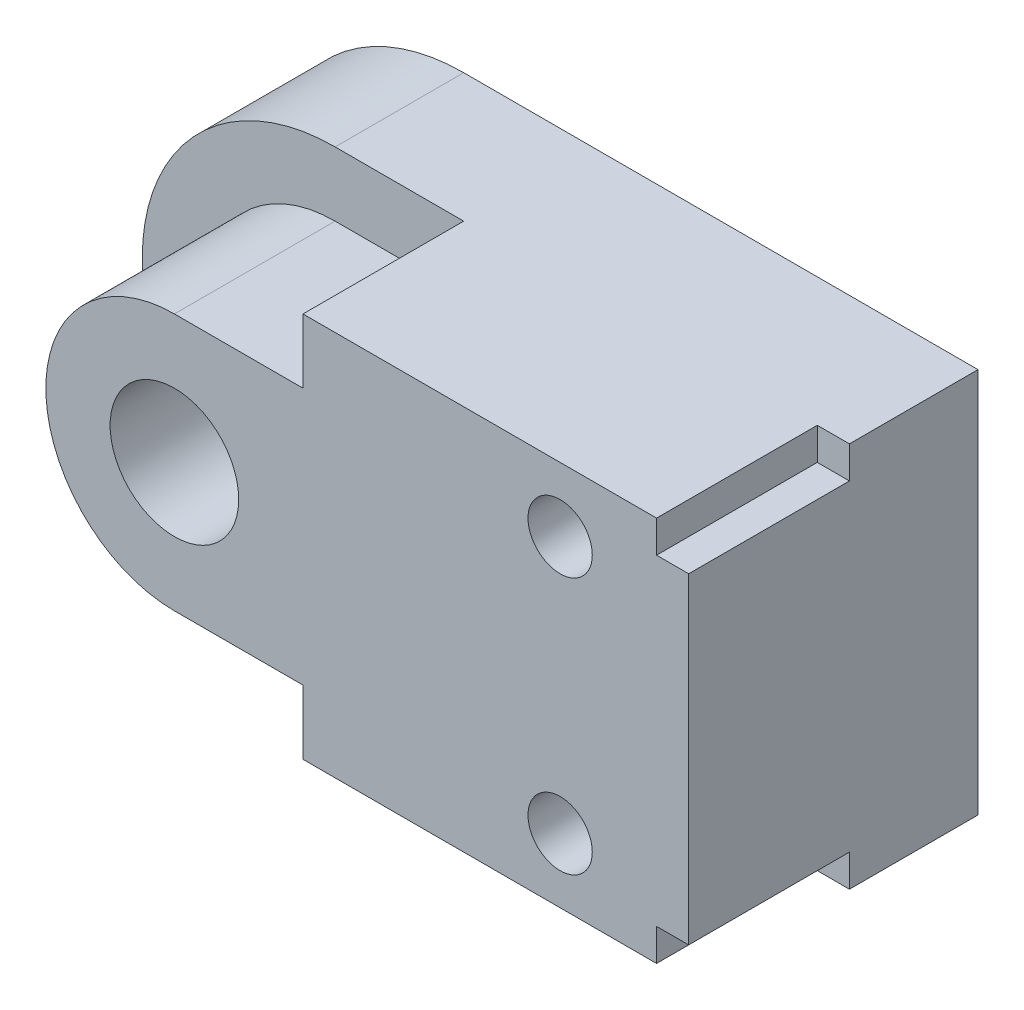
ISO-10303-21;
HEADER;
FILE_DESCRIPTION(('STEP AP214'),'2;1');
FILE_NAME('part.step','',(''),(''),'','','');
FILE_SCHEMA(('AUTOMOTIVE_DESIGN { 1 0 10303 214 1 1 1 1 }'));
ENDSEC;
DATA;
#1=APPLICATION_CONTEXT('core data for automotive mechanical design processes');
#2=APPLICATION_PROTOCOL_DEFINITION('international standard','automotive_design',2000,#1);
#3=PRODUCT_CONTEXT('',#1,'mechanical');
#4=PRODUCT('Part','Part','',(#3));
#5=PRODUCT_RELATED_PRODUCT_CATEGORY('part','',(#4));
#6=PRODUCT_DEFINITION_FORMATION('','',#4);
#7=PRODUCT_DEFINITION_CONTEXT('part definition',#1,'design');
#8=PRODUCT_DEFINITION('design','',#6,#7);
#9=PRODUCT_DEFINITION_SHAPE('','',#8);
#10=(LENGTH_UNIT() NAMED_UNIT(*) SI_UNIT(.MILLI.,.METRE.));
#11=(NAMED_UNIT(*) PLANE_ANGLE_UNIT() SI_UNIT($,.RADIAN.));
#12=(NAMED_UNIT(*) SI_UNIT($,.STERADIAN.) SOLID_ANGLE_UNIT());
#13=UNCERTAINTY_MEASURE_WITH_UNIT(LENGTH_MEASURE(1.E-05),#10,'distance_accuracy_value','');
#14=(GEOMETRIC_REPRESENTATION_CONTEXT(3) GLOBAL_UNCERTAINTY_ASSIGNED_CONTEXT((#13)) GLOBAL_UNIT_ASSIGNED_CONTEXT((#10,
#11,#12)) REPRESENTATION_CONTEXT('',''));
#15=CARTESIAN_POINT('',(0.,0.,0.));
#16=DIRECTION('',(0.,0.,1.));
#17=DIRECTION('',(1.,0.,0.));
#18=AXIS2_PLACEMENT_3D('',#15,#16,#17);
#19=CARTESIAN_POINT('',(0.,0.,20.));
#20=DIRECTION('',(0.,0.,1.));
#21=DIRECTION('',(1.,0.,0.));
#22=AXIS2_PLACEMENT_3D('',#19,#20,#21);
#23=PLANE('',#22);
#24=DIRECTION('',(0.,1.,0.));
#25=VECTOR('',#24,1.);
#26=CARTESIAN_POINT('',(75.,30.,20.));
#27=LINE('',#26,#25);
#28=CARTESIAN_POINT('',(75.,25.,20.));
#29=VERTEX_POINT('',#28);
#30=CARTESIAN_POINT('',(75.,30.,20.));
#31=VERTEX_POINT('',#30);
#32=EDGE_CURVE('E53',#29,#31,#27,.T.);
#33=ORIENTED_EDGE('',*,*,#32,.F.);
#34=DIRECTION('',(-1.,0.,0.));
#35=VECTOR('',#34,1.);
#36=CARTESIAN_POINT('',(80.,25.,20.));
#37=LINE('',#36,#35);
#38=CARTESIAN_POINT('',(80.,25.,20.));
#39=VERTEX_POINT('',#38);
#40=EDGE_CURVE('E288',#39,#29,#37,.T.);
#41=ORIENTED_EDGE('',*,*,#40,.F.);
#42=DIRECTION('',(0.,1.,0.));
#43=VECTOR('',#42,1.);
#44=CARTESIAN_POINT('',(80.,30.,20.));
#45=LINE('',#44,#43);
#46=CARTESIAN_POINT('',(80.,30.,20.));
#47=VERTEX_POINT('',#46);
#48=EDGE_CURVE('E193',#39,#47,#45,.T.);
#49=ORIENTED_EDGE('',*,*,#48,.T.);
#50=DIRECTION('',(-1.,0.,0.));
#51=VECTOR('',#50,1.);
#52=CARTESIAN_POINT('',(0.,30.,20.));
#53=LINE('',#52,#51);
#54=EDGE_CURVE('E196',#47,#31,#53,.T.);
#55=ORIENTED_EDGE('',*,*,#54,.T.);
#56=EDGE_LOOP('',(#33,#41,#49,#55));
#57=FACE_BOUND('',#56,.T.);
#58=ADVANCED_FACE('F39',(#57),#23,.T.);
#59=DIRECTION('',(1.,0.,0.));
#60=VECTOR('',#59,1.);
#61=CARTESIAN_POINT('',(80.,-25.,20.));
#62=LINE('',#61,#60);
#63=CARTESIAN_POINT('',(75.,-25.,20.));
#64=VERTEX_POINT('',#63);
#65=CARTESIAN_POINT('',(80.,-25.,20.));
#66=VERTEX_POINT('',#65);
#67=EDGE_CURVE('E64',#64,#66,#62,.T.);
#68=ORIENTED_EDGE('',*,*,#67,.F.);
#69=DIRECTION('',(0.,1.,0.));
#70=VECTOR('',#69,1.);
#71=CARTESIAN_POINT('',(75.,-30.,20.));
#72=LINE('',#71,#70);
#73=CARTESIAN_POINT('',(75.,-30.,20.));
#74=VERTEX_POINT('',#73);
#75=EDGE_CURVE('E283',#74,#64,#72,.T.);
#76=ORIENTED_EDGE('',*,*,#75,.F.);
#77=DIRECTION('',(1.,0.,0.));
#78=VECTOR('',#77,1.);
#79=CARTESIAN_POINT('',(80.,-30.,20.));
#80=LINE('',#79,#78);
#81=CARTESIAN_POINT('',(80.,-30.,20.));
#82=VERTEX_POINT('',#81);
#83=EDGE_CURVE('E186',#74,#82,#80,.T.);
#84=ORIENTED_EDGE('',*,*,#83,.T.);
#85=EDGE_CURVE('E192',#82,#66,#45,.T.);
#86=ORIENTED_EDGE('',*,*,#85,.T.);
#87=EDGE_LOOP('',(#68,#76,#84,#86));
#88=FACE_BOUND('',#87,.T.);
#89=ADVANCED_FACE('F340',(#88),#23,.T.);
#90=DIRECTION('',(0.,-1.,0.));
#91=VECTOR('',#90,1.);
#92=CARTESIAN_POINT('',(20.,20.,20.));
#93=LINE('',#92,#91);
#94=CARTESIAN_POINT('',(20.,30.,20.));
#95=VERTEX_POINT('',#94);
#96=CARTESIAN_POINT('',(20.,20.,20.));
#97=VERTEX_POINT('',#96);
#98=EDGE_CURVE('E239',#95,#97,#93,.T.);
#99=ORIENTED_EDGE('',*,*,#98,.F.);
#100=CARTESIAN_POINT('',(0.,30.,20.));
#101=VERTEX_POINT('',#100);
#102=EDGE_CURVE('E197',#95,#101,#53,.T.);
#103=ORIENTED_EDGE('',*,*,#102,.T.);
#104=CARTESIAN_POINT('',(0.,0.,20.));
#105=DIRECTION('',(0.,0.,1.));
#106=DIRECTION('',(1.,0.,0.));
#107=AXIS2_PLACEMENT_3D('',#104,#105,#106);
#108=CIRCLE('',#107,30.);
#109=CARTESIAN_POINT('',(0.,-30.,20.));
#110=VERTEX_POINT('',#109);
#111=EDGE_CURVE('E189',#101,#110,#108,.T.);
#112=ORIENTED_EDGE('',*,*,#111,.T.);
#113=CARTESIAN_POINT('',(20.,-30.,20.));
#114=VERTEX_POINT('',#113);
#115=EDGE_CURVE('E191',#110,#114,#80,.T.);
#116=ORIENTED_EDGE('',*,*,#115,.T.);
#117=DIRECTION('',(0.,-1.,0.));
#118=VECTOR('',#117,1.);
#119=CARTESIAN_POINT('',(20.,-30.,20.));
#120=LINE('',#119,#118);
#121=CARTESIAN_POINT('',(20.,-20.,20.));
#122=VERTEX_POINT('',#121);
#123=EDGE_CURVE('E278',#122,#114,#120,.T.);
#124=ORIENTED_EDGE('',*,*,#123,.F.);
#125=DIRECTION('',(1.,0.,0.));
#126=VECTOR('',#125,1.);
#127=CARTESIAN_POINT('',(20.,-20.,20.));
#128=LINE('',#127,#126);
#129=CARTESIAN_POINT('',(0.,-20.,20.));
#130=VERTEX_POINT('',#129);
#131=EDGE_CURVE('E284',#130,#122,#128,.T.);
#132=ORIENTED_EDGE('',*,*,#131,.F.);
#133=CARTESIAN_POINT('',(0.,0.,20.));
#134=DIRECTION('',(0.,0.,1.));
#135=DIRECTION('',(1.,0.,0.));
#136=AXIS2_PLACEMENT_3D('',#133,#134,#135);
#137=CIRCLE('',#136,20.);
#138=CARTESIAN_POINT('',(0.,20.,20.));
#139=VERTEX_POINT('',#138);
#140=EDGE_CURVE('E176',#139,#130,#137,.T.);
#141=ORIENTED_EDGE('',*,*,#140,.F.);
#142=DIRECTION('',(-1.,0.,0.));
#143=VECTOR('',#142,1.);
#144=CARTESIAN_POINT('',(0.,20.,20.));
#145=LINE('',#144,#143);
#146=EDGE_CURVE('E175',#97,#139,#145,.T.);
#147=ORIENTED_EDGE('',*,*,#146,.F.);
#148=EDGE_LOOP('',(#99,#103,#112,#116,#124,#132,#141,#147));
#149=FACE_BOUND('',#148,.T.);
#150=ADVANCED_FACE('F237',(#149),#23,.T.);
#151=CARTESIAN_POINT('',(0.,0.,0.));
#152=DIRECTION('',(0.,0.,1.));
#153=DIRECTION('',(1.,0.,0.));
#154=AXIS2_PLACEMENT_3D('',#151,#152,#153);
#155=PLANE('',#154);
#156=CARTESIAN_POINT('',(60.,-20.,0.));
#157=DIRECTION('',(0.,0.,1.));
#158=DIRECTION('',(1.,0.,0.));
#159=AXIS2_PLACEMENT_3D('',#156,#157,#158);
#160=CIRCLE('',#159,5.);
#161=CARTESIAN_POINT('',(65.,-20.,0.));
#162=VERTEX_POINT('',#161);
#163=EDGE_CURVE('E540',#162,#162,#160,.T.);
#164=ORIENTED_EDGE('',*,*,#163,.T.);
#165=EDGE_LOOP('',(#164));
#166=FACE_BOUND('',#165,.T.);
#167=CARTESIAN_POINT('',(60.,20.,0.));
#168=DIRECTION('',(0.,0.,1.));
#169=DIRECTION('',(1.,0.,0.));
#170=AXIS2_PLACEMENT_3D('',#167,#168,#169);
#171=CIRCLE('',#170,5.);
#172=CARTESIAN_POINT('',(65.,20.,0.));
#173=VERTEX_POINT('',#172);
#174=EDGE_CURVE('E538',#173,#173,#171,.T.);
#175=ORIENTED_EDGE('',*,*,#174,.T.);
#176=EDGE_LOOP('',(#175));
#177=FACE_BOUND('',#176,.T.);
#178=CARTESIAN_POINT('',(0.,0.,0.));
#179=DIRECTION('',(0.,0.,1.));
#180=DIRECTION('',(1.,0.,0.));
#181=AXIS2_PLACEMENT_3D('',#178,#179,#180);
#182=CIRCLE('',#181,30.);
#183=CARTESIAN_POINT('',(0.,30.,0.));
#184=VERTEX_POINT('',#183);
#185=CARTESIAN_POINT('',(0.,-30.,0.));
#186=VERTEX_POINT('',#185);
#187=EDGE_CURVE('E182',#184,#186,#182,.T.);
#188=ORIENTED_EDGE('',*,*,#187,.F.);
#189=DIRECTION('',(-1.,0.,0.));
#190=VECTOR('',#189,1.);
#191=CARTESIAN_POINT('',(0.,30.,0.));
#192=LINE('',#191,#190);
#193=CARTESIAN_POINT('',(80.,30.,0.));
#194=VERTEX_POINT('',#193);
#195=EDGE_CURVE('E194',#194,#184,#192,.T.);
#196=ORIENTED_EDGE('',*,*,#195,.F.);
#197=DIRECTION('',(0.,1.,0.));
#198=VECTOR('',#197,1.);
#199=CARTESIAN_POINT('',(80.,30.,0.));
#200=LINE('',#199,#198);
#201=CARTESIAN_POINT('',(80.,-30.,0.));
#202=VERTEX_POINT('',#201);
#203=EDGE_CURVE('E202',#202,#194,#200,.T.);
#204=ORIENTED_EDGE('',*,*,#203,.F.);
#205=DIRECTION('',(1.,0.,0.));
#206=VECTOR('',#205,1.);
#207=CARTESIAN_POINT('',(80.,-30.,0.));
#208=LINE('',#207,#206);
#209=EDGE_CURVE('E201',#186,#202,#208,.T.);
#210=ORIENTED_EDGE('',*,*,#209,.F.);
#211=EDGE_LOOP('',(#188,#196,#204,#210));
#212=FACE_BOUND('',#211,.T.);
#213=CARTESIAN_POINT('',(0.,0.,0.));
#214=DIRECTION('',(0.,0.,1.));
#215=DIRECTION('',(1.,0.,0.));
#216=AXIS2_PLACEMENT_3D('',#213,#214,#215);
#217=CIRCLE('',#216,10.);
#218=CARTESIAN_POINT('',(10.,0.,0.));
#219=VERTEX_POINT('',#218);
#220=EDGE_CURVE('E180',#219,#219,#217,.T.);
#221=ORIENTED_EDGE('',*,*,#220,.T.);
#222=EDGE_LOOP('',(#221));
#223=FACE_BOUND('',#222,.T.);
#224=ADVANCED_FACE('F223',(#166,#177,#212,#223),#155,.F.);
#225=CARTESIAN_POINT('',(0.,0.,20.));
#226=DIRECTION('',(0.,0.,-1.));
#227=DIRECTION('',(-1.,0.,0.));
#228=AXIS2_PLACEMENT_3D('',#225,#226,#227);
#229=CYLINDRICAL_SURFACE('',#228,30.);
#230=ORIENTED_EDGE('',*,*,#187,.T.);
#231=DIRECTION('',(0.,0.,-1.));
#232=VECTOR('',#231,1.);
#233=CARTESIAN_POINT('',(0.,-30.,20.));
#234=LINE('',#233,#232);
#235=EDGE_CURVE('E11',#110,#186,#234,.T.);
#236=ORIENTED_EDGE('',*,*,#235,.F.);
#237=ORIENTED_EDGE('',*,*,#111,.F.);
#238=DIRECTION('',(0.,0.,-1.));
#239=VECTOR('',#238,1.);
#240=CARTESIAN_POINT('',(0.,30.,20.));
#241=LINE('',#240,#239);
#242=EDGE_CURVE('E199',#101,#184,#241,.T.);
#243=ORIENTED_EDGE('',*,*,#242,.T.);
#244=EDGE_LOOP('',(#230,#236,#237,#243));
#245=FACE_BOUND('',#244,.T.);
#246=ADVANCED_FACE('F41',(#245),#229,.T.);
#247=CARTESIAN_POINT('',(80.,-30.,20.));
#248=DIRECTION('',(0.,1.,0.));
#249=DIRECTION('',(-1.,0.,0.));
#250=AXIS2_PLACEMENT_3D('',#247,#248,#249);
#251=PLANE('',#250);
#252=ORIENTED_EDGE('',*,*,#209,.T.);
#253=DIRECTION('',(0.,0.,-1.));
#254=VECTOR('',#253,1.);
#255=CARTESIAN_POINT('',(80.,-30.,20.));
#256=LINE('',#255,#254);
#257=EDGE_CURVE('E50',#82,#202,#256,.T.);
#258=ORIENTED_EDGE('',*,*,#257,.F.);
#259=ORIENTED_EDGE('',*,*,#83,.F.);
#260=DIRECTION('',(0.,0.,-1.));
#261=VECTOR('',#260,1.);
#262=CARTESIAN_POINT('',(75.,-30.,45.));
#263=LINE('',#262,#261);
#264=CARTESIAN_POINT('',(75.,-30.,45.));
#265=VERTEX_POINT('',#264);
#266=EDGE_CURVE('E269',#265,#74,#263,.T.);
#267=ORIENTED_EDGE('',*,*,#266,.F.);
#268=DIRECTION('',(1.,0.,0.));
#269=VECTOR('',#268,1.);
#270=CARTESIAN_POINT('',(75.,-30.,45.));
#271=LINE('',#270,#269);
#272=CARTESIAN_POINT('',(20.,-30.,45.));
#273=VERTEX_POINT('',#272);
#274=EDGE_CURVE('E280',#273,#265,#271,.T.);
#275=ORIENTED_EDGE('',*,*,#274,.F.);
#276=DIRECTION('',(0.,0.,-1.));
#277=VECTOR('',#276,1.);
#278=CARTESIAN_POINT('',(20.,-30.,45.));
#279=LINE('',#278,#277);
#280=EDGE_CURVE('E181',#273,#114,#279,.T.);
#281=ORIENTED_EDGE('',*,*,#280,.T.);
#282=ORIENTED_EDGE('',*,*,#115,.F.);
#283=ORIENTED_EDGE('',*,*,#235,.T.);
#284=EDGE_LOOP('',(#252,#258,#259,#267,#275,#281,#282,#283));
#285=FACE_BOUND('',#284,.T.);
#286=ADVANCED_FACE('F274',(#285),#251,.F.);
#287=CARTESIAN_POINT('',(80.,30.,20.));
#288=DIRECTION('',(-1.,0.,0.));
#289=DIRECTION('',(0.,0.,1.));
#290=AXIS2_PLACEMENT_3D('',#287,#288,#289);
#291=PLANE('',#290);
#292=ORIENTED_EDGE('',*,*,#203,.T.);
#293=DIRECTION('',(0.,0.,-1.));
#294=VECTOR('',#293,1.);
#295=CARTESIAN_POINT('',(80.,30.,20.));
#296=LINE('',#295,#294);
#297=EDGE_CURVE('E209',#47,#194,#296,.T.);
#298=ORIENTED_EDGE('',*,*,#297,.F.);
#299=ORIENTED_EDGE('',*,*,#48,.F.);
#300=DIRECTION('',(0.,0.,-1.));
#301=VECTOR('',#300,1.);
#302=CARTESIAN_POINT('',(80.,25.,45.));
#303=LINE('',#302,#301);
#304=CARTESIAN_POINT('',(80.,25.,45.));
#305=VERTEX_POINT('',#304);
#306=EDGE_CURVE('E265',#305,#39,#303,.T.);
#307=ORIENTED_EDGE('',*,*,#306,.F.);
#308=DIRECTION('',(0.,1.,0.));
#309=VECTOR('',#308,1.);
#310=CARTESIAN_POINT('',(80.,25.,45.));
#311=LINE('',#310,#309);
#312=CARTESIAN_POINT('',(80.,-25.,45.));
#313=VERTEX_POINT('',#312);
#314=EDGE_CURVE('E312',#313,#305,#311,.T.);
#315=ORIENTED_EDGE('',*,*,#314,.F.);
#316=DIRECTION('',(0.,0.,-1.));
#317=VECTOR('',#316,1.);
#318=CARTESIAN_POINT('',(80.,-25.,45.));
#319=LINE('',#318,#317);
#320=EDGE_CURVE('E264',#313,#66,#319,.T.);
#321=ORIENTED_EDGE('',*,*,#320,.T.);
#322=ORIENTED_EDGE('',*,*,#85,.F.);
#323=ORIENTED_EDGE('',*,*,#257,.T.);
#324=EDGE_LOOP('',(#292,#298,#299,#307,#315,#321,#322,#323));
#325=FACE_BOUND('',#324,.T.);
#326=ADVANCED_FACE('F220',(#325),#291,.F.);
#327=CARTESIAN_POINT('',(0.,30.,20.));
#328=DIRECTION('',(0.,-1.,0.));
#329=DIRECTION('',(1.,0.,0.));
#330=AXIS2_PLACEMENT_3D('',#327,#328,#329);
#331=PLANE('',#330);
#332=ORIENTED_EDGE('',*,*,#195,.T.);
#333=ORIENTED_EDGE('',*,*,#242,.F.);
#334=ORIENTED_EDGE('',*,*,#102,.F.);
#335=DIRECTION('',(0.,0.,-1.));
#336=VECTOR('',#335,1.);
#337=CARTESIAN_POINT('',(20.,30.,45.));
#338=LINE('',#337,#336);
#339=CARTESIAN_POINT('',(20.,30.,45.));
#340=VERTEX_POINT('',#339);
#341=EDGE_CURVE('E242',#340,#95,#338,.T.);
#342=ORIENTED_EDGE('',*,*,#341,.F.);
#343=DIRECTION('',(-1.,0.,0.));
#344=VECTOR('',#343,1.);
#345=CARTESIAN_POINT('',(20.,30.,45.));
#346=LINE('',#345,#344);
#347=CARTESIAN_POINT('',(75.,30.,45.));
#348=VERTEX_POINT('',#347);
#349=EDGE_CURVE('E293',#348,#340,#346,.T.);
#350=ORIENTED_EDGE('',*,*,#349,.F.);
#351=DIRECTION('',(0.,0.,-1.));
#352=VECTOR('',#351,1.);
#353=CARTESIAN_POINT('',(75.,30.,45.));
#354=LINE('',#353,#352);
#355=EDGE_CURVE('E247',#348,#31,#354,.T.);
#356=ORIENTED_EDGE('',*,*,#355,.T.);
#357=ORIENTED_EDGE('',*,*,#54,.F.);
#358=ORIENTED_EDGE('',*,*,#297,.T.);
#359=EDGE_LOOP('',(#332,#333,#334,#342,#350,#356,#357,#358));
#360=FACE_BOUND('',#359,.T.);
#361=ADVANCED_FACE('F230',(#360),#331,.F.);
#362=CARTESIAN_POINT('',(0.,0.,20.));
#363=DIRECTION('',(0.,0.,-1.));
#364=DIRECTION('',(-1.,0.,0.));
#365=AXIS2_PLACEMENT_3D('',#362,#363,#364);
#366=CYLINDRICAL_SURFACE('',#365,10.);
#367=ORIENTED_EDGE('',*,*,#220,.F.);
#368=EDGE_LOOP('',(#367));
#369=FACE_BOUND('',#368,.T.);
#370=CARTESIAN_POINT('',(0.,0.,45.));
#371=DIRECTION('',(0.,0.,1.));
#372=DIRECTION('',(1.,0.,0.));
#373=AXIS2_PLACEMENT_3D('',#370,#371,#372);
#374=CIRCLE('',#373,10.);
#375=CARTESIAN_POINT('',(10.,0.,45.));
#376=VERTEX_POINT('',#375);
#377=EDGE_CURVE('E297',#376,#376,#374,.T.);
#378=ORIENTED_EDGE('',*,*,#377,.T.);
#379=EDGE_LOOP('',(#378));
#380=FACE_BOUND('',#379,.T.);
#381=ADVANCED_FACE('F346',(#369,#380),#366,.F.);
#382=CARTESIAN_POINT('',(0.,0.,45.));
#383=DIRECTION('',(0.,0.,1.));
#384=DIRECTION('',(1.,0.,0.));
#385=AXIS2_PLACEMENT_3D('',#382,#383,#384);
#386=PLANE('',#385);
#387=CARTESIAN_POINT('',(60.,20.,45.));
#388=DIRECTION('',(0.,0.,1.));
#389=DIRECTION('',(1.,0.,0.));
#390=AXIS2_PLACEMENT_3D('',#387,#388,#389);
#391=CIRCLE('',#390,5.);
#392=CARTESIAN_POINT('',(65.,20.,45.));
#393=VERTEX_POINT('',#392);
#394=EDGE_CURVE('E296',#393,#393,#391,.T.);
#395=ORIENTED_EDGE('',*,*,#394,.F.);
#396=EDGE_LOOP('',(#395));
#397=FACE_BOUND('',#396,.T.);
#398=CARTESIAN_POINT('',(0.,0.,45.));
#399=DIRECTION('',(0.,0.,1.));
#400=DIRECTION('',(1.,0.,0.));
#401=AXIS2_PLACEMENT_3D('',#398,#399,#400);
#402=CIRCLE('',#401,20.);
#403=CARTESIAN_POINT('',(0.,20.,45.));
#404=VERTEX_POINT('',#403);
#405=CARTESIAN_POINT('',(0.,-20.,45.));
#406=VERTEX_POINT('',#405);
#407=EDGE_CURVE('E163',#404,#406,#402,.T.);
#408=ORIENTED_EDGE('',*,*,#407,.T.);
#409=DIRECTION('',(1.,0.,0.));
#410=VECTOR('',#409,1.);
#411=CARTESIAN_POINT('',(20.,-20.,45.));
#412=LINE('',#411,#410);
#413=CARTESIAN_POINT('',(20.,-20.,45.));
#414=VERTEX_POINT('',#413);
#415=EDGE_CURVE('E155',#406,#414,#412,.T.);
#416=ORIENTED_EDGE('',*,*,#415,.T.);
#417=DIRECTION('',(0.,-1.,0.));
#418=VECTOR('',#417,1.);
#419=CARTESIAN_POINT('',(20.,-30.,45.));
#420=LINE('',#419,#418);
#421=EDGE_CURVE('E162',#414,#273,#420,.T.);
#422=ORIENTED_EDGE('',*,*,#421,.T.);
#423=ORIENTED_EDGE('',*,*,#274,.T.);
#424=DIRECTION('',(0.,1.,0.));
#425=VECTOR('',#424,1.);
#426=CARTESIAN_POINT('',(75.,-30.,45.));
#427=LINE('',#426,#425);
#428=CARTESIAN_POINT('',(75.,-25.,45.));
#429=VERTEX_POINT('',#428);
#430=EDGE_CURVE('E313',#265,#429,#427,.T.);
#431=ORIENTED_EDGE('',*,*,#430,.T.);
#432=DIRECTION('',(1.,0.,0.));
#433=VECTOR('',#432,1.);
#434=CARTESIAN_POINT('',(80.,-25.,45.));
#435=LINE('',#434,#433);
#436=EDGE_CURVE('E311',#429,#313,#435,.T.);
#437=ORIENTED_EDGE('',*,*,#436,.T.);
#438=ORIENTED_EDGE('',*,*,#314,.T.);
#439=DIRECTION('',(-1.,0.,0.));
#440=VECTOR('',#439,1.);
#441=CARTESIAN_POINT('',(80.,25.,45.));
#442=LINE('',#441,#440);
#443=CARTESIAN_POINT('',(75.,25.,45.));
#444=VERTEX_POINT('',#443);
#445=EDGE_CURVE('E320',#305,#444,#442,.T.);
#446=ORIENTED_EDGE('',*,*,#445,.T.);
#447=DIRECTION('',(0.,1.,0.));
#448=VECTOR('',#447,1.);
#449=CARTESIAN_POINT('',(75.,30.,45.));
#450=LINE('',#449,#448);
#451=EDGE_CURVE('E317',#444,#348,#450,.T.);
#452=ORIENTED_EDGE('',*,*,#451,.T.);
#453=ORIENTED_EDGE('',*,*,#349,.T.);
#454=DIRECTION('',(0.,-1.,0.));
#455=VECTOR('',#454,1.);
#456=CARTESIAN_POINT('',(20.,20.,45.));
#457=LINE('',#456,#455);
#458=CARTESIAN_POINT('',(20.,20.,45.));
#459=VERTEX_POINT('',#458);
#460=EDGE_CURVE('E248',#340,#459,#457,.T.);
#461=ORIENTED_EDGE('',*,*,#460,.T.);
#462=DIRECTION('',(-1.,0.,0.));
#463=VECTOR('',#462,1.);
#464=CARTESIAN_POINT('',(0.,20.,45.));
#465=LINE('',#464,#463);
#466=EDGE_CURVE('E168',#459,#404,#465,.T.);
#467=ORIENTED_EDGE('',*,*,#466,.T.);
#468=EDGE_LOOP('',(#408,#416,#422,#423,#431,#437,#438,#446,#452,#453,#461,#467));
#469=FACE_BOUND('',#468,.T.);
#470=ORIENTED_EDGE('',*,*,#377,.F.);
#471=EDGE_LOOP('',(#470));
#472=FACE_BOUND('',#471,.T.);
#473=CARTESIAN_POINT('',(60.,-20.,45.));
#474=DIRECTION('',(0.,0.,1.));
#475=DIRECTION('',(1.,0.,0.));
#476=AXIS2_PLACEMENT_3D('',#473,#474,#475);
#477=CIRCLE('',#476,5.);
#478=CARTESIAN_POINT('',(65.,-20.,45.));
#479=VERTEX_POINT('',#478);
#480=EDGE_CURVE('E302',#479,#479,#477,.T.);
#481=ORIENTED_EDGE('',*,*,#480,.F.);
#482=EDGE_LOOP('',(#481));
#483=FACE_BOUND('',#482,.T.);
#484=ADVANCED_FACE('F170',(#397,#469,#472,#483),#386,.T.);
#485=CARTESIAN_POINT('',(0.,0.,45.));
#486=DIRECTION('',(0.,0.,-1.));
#487=DIRECTION('',(-1.,0.,0.));
#488=AXIS2_PLACEMENT_3D('',#485,#486,#487);
#489=CYLINDRICAL_SURFACE('',#488,20.);
#490=ORIENTED_EDGE('',*,*,#140,.T.);
#491=DIRECTION('',(0.,0.,-1.));
#492=VECTOR('',#491,1.);
#493=CARTESIAN_POINT('',(0.,-20.,45.));
#494=LINE('',#493,#492);
#495=EDGE_CURVE('E160',#406,#130,#494,.T.);
#496=ORIENTED_EDGE('',*,*,#495,.F.);
#497=ORIENTED_EDGE('',*,*,#407,.F.);
#498=DIRECTION('',(0.,0.,-1.));
#499=VECTOR('',#498,1.);
#500=CARTESIAN_POINT('',(0.,20.,45.));
#501=LINE('',#500,#499);
#502=EDGE_CURVE('E258',#404,#139,#501,.T.);
#503=ORIENTED_EDGE('',*,*,#502,.T.);
#504=EDGE_LOOP('',(#490,#496,#497,#503));
#505=FACE_BOUND('',#504,.T.);
#506=ADVANCED_FACE('F179',(#505),#489,.T.);
#507=CARTESIAN_POINT('',(20.,-20.,45.));
#508=DIRECTION('',(0.,1.,0.));
#509=DIRECTION('',(0.,0.,1.));
#510=AXIS2_PLACEMENT_3D('',#507,#508,#509);
#511=PLANE('',#510);
#512=ORIENTED_EDGE('',*,*,#131,.T.);
#513=DIRECTION('',(0.,0.,-1.));
#514=VECTOR('',#513,1.);
#515=CARTESIAN_POINT('',(20.,-20.,45.));
#516=LINE('',#515,#514);
#517=EDGE_CURVE('E159',#414,#122,#516,.T.);
#518=ORIENTED_EDGE('',*,*,#517,.F.);
#519=ORIENTED_EDGE('',*,*,#415,.F.);
#520=ORIENTED_EDGE('',*,*,#495,.T.);
#521=EDGE_LOOP('',(#512,#518,#519,#520));
#522=FACE_BOUND('',#521,.T.);
#523=ADVANCED_FACE('F154',(#522),#511,.F.);
#524=CARTESIAN_POINT('',(20.,-30.,45.));
#525=DIRECTION('',(1.,0.,0.));
#526=DIRECTION('',(0.,0.,-1.));
#527=AXIS2_PLACEMENT_3D('',#524,#525,#526);
#528=PLANE('',#527);
#529=ORIENTED_EDGE('',*,*,#123,.T.);
#530=ORIENTED_EDGE('',*,*,#280,.F.);
#531=ORIENTED_EDGE('',*,*,#421,.F.);
#532=ORIENTED_EDGE('',*,*,#517,.T.);
#533=EDGE_LOOP('',(#529,#530,#531,#532));
#534=FACE_BOUND('',#533,.T.);
#535=ADVANCED_FACE('F276',(#534),#528,.F.);
#536=CARTESIAN_POINT('',(75.,-30.,45.));
#537=DIRECTION('',(-1.,0.,0.));
#538=DIRECTION('',(0.,0.,1.));
#539=AXIS2_PLACEMENT_3D('',#536,#537,#538);
#540=PLANE('',#539);
#541=ORIENTED_EDGE('',*,*,#75,.T.);
#542=DIRECTION('',(0.,0.,-1.));
#543=VECTOR('',#542,1.);
#544=CARTESIAN_POINT('',(75.,-25.,45.));
#545=LINE('',#544,#543);
#546=EDGE_CURVE('E270',#429,#64,#545,.T.);
#547=ORIENTED_EDGE('',*,*,#546,.F.);
#548=ORIENTED_EDGE('',*,*,#430,.F.);
#549=ORIENTED_EDGE('',*,*,#266,.T.);
#550=EDGE_LOOP('',(#541,#547,#548,#549));
#551=FACE_BOUND('',#550,.T.);
#552=ADVANCED_FACE('F337',(#551),#540,.F.);
#553=CARTESIAN_POINT('',(80.,-25.,45.));
#554=DIRECTION('',(0.,1.,0.));
#555=DIRECTION('',(0.,0.,1.));
#556=AXIS2_PLACEMENT_3D('',#553,#554,#555);
#557=PLANE('',#556);
#558=ORIENTED_EDGE('',*,*,#67,.T.);
#559=ORIENTED_EDGE('',*,*,#320,.F.);
#560=ORIENTED_EDGE('',*,*,#436,.F.);
#561=ORIENTED_EDGE('',*,*,#546,.T.);
#562=EDGE_LOOP('',(#558,#559,#560,#561));
#563=FACE_BOUND('',#562,.T.);
#564=ADVANCED_FACE('F338',(#563),#557,.F.);
#565=CARTESIAN_POINT('',(80.,25.,45.));
#566=DIRECTION('',(0.,-1.,0.));
#567=DIRECTION('',(0.,0.,-1.));
#568=AXIS2_PLACEMENT_3D('',#565,#566,#567);
#569=PLANE('',#568);
#570=ORIENTED_EDGE('',*,*,#40,.T.);
#571=DIRECTION('',(0.,0.,-1.));
#572=VECTOR('',#571,1.);
#573=CARTESIAN_POINT('',(75.,25.,45.));
#574=LINE('',#573,#572);
#575=EDGE_CURVE('E255',#444,#29,#574,.T.);
#576=ORIENTED_EDGE('',*,*,#575,.F.);
#577=ORIENTED_EDGE('',*,*,#445,.F.);
#578=ORIENTED_EDGE('',*,*,#306,.T.);
#579=EDGE_LOOP('',(#570,#576,#577,#578));
#580=FACE_BOUND('',#579,.T.);
#581=ADVANCED_FACE('F330',(#580),#569,.F.);
#582=CARTESIAN_POINT('',(75.,30.,45.));
#583=DIRECTION('',(-1.,0.,0.));
#584=DIRECTION('',(0.,0.,1.));
#585=AXIS2_PLACEMENT_3D('',#582,#583,#584);
#586=PLANE('',#585);
#587=ORIENTED_EDGE('',*,*,#32,.T.);
#588=ORIENTED_EDGE('',*,*,#355,.F.);
#589=ORIENTED_EDGE('',*,*,#451,.F.);
#590=ORIENTED_EDGE('',*,*,#575,.T.);
#591=EDGE_LOOP('',(#587,#588,#589,#590));
#592=FACE_BOUND('',#591,.T.);
#593=ADVANCED_FACE('F323',(#592),#586,.F.);
#594=CARTESIAN_POINT('',(20.,20.,45.));
#595=DIRECTION('',(1.,0.,0.));
#596=DIRECTION('',(0.,1.,0.));
#597=AXIS2_PLACEMENT_3D('',#594,#595,#596);
#598=PLANE('',#597);
#599=ORIENTED_EDGE('',*,*,#98,.T.);
#600=DIRECTION('',(0.,0.,-1.));
#601=VECTOR('',#600,1.);
#602=CARTESIAN_POINT('',(20.,20.,45.));
#603=LINE('',#602,#601);
#604=EDGE_CURVE('E253',#459,#97,#603,.T.);
#605=ORIENTED_EDGE('',*,*,#604,.F.);
#606=ORIENTED_EDGE('',*,*,#460,.F.);
#607=ORIENTED_EDGE('',*,*,#341,.T.);
#608=EDGE_LOOP('',(#599,#605,#606,#607));
#609=FACE_BOUND('',#608,.T.);
#610=ADVANCED_FACE('F249',(#609),#598,.F.);
#611=CARTESIAN_POINT('',(0.,20.,45.));
#612=DIRECTION('',(0.,-1.,0.));
#613=DIRECTION('',(0.,0.,-1.));
#614=AXIS2_PLACEMENT_3D('',#611,#612,#613);
#615=PLANE('',#614);
#616=ORIENTED_EDGE('',*,*,#146,.T.);
#617=ORIENTED_EDGE('',*,*,#502,.F.);
#618=ORIENTED_EDGE('',*,*,#466,.F.);
#619=ORIENTED_EDGE('',*,*,#604,.T.);
#620=EDGE_LOOP('',(#616,#617,#618,#619));
#621=FACE_BOUND('',#620,.T.);
#622=ADVANCED_FACE('F480',(#621),#615,.F.);
#623=CARTESIAN_POINT('',(60.,20.,45.));
#624=DIRECTION('',(0.,0.,-1.));
#625=DIRECTION('',(-1.,0.,0.));
#626=AXIS2_PLACEMENT_3D('',#623,#624,#625);
#627=CYLINDRICAL_SURFACE('',#626,5.);
#628=ORIENTED_EDGE('',*,*,#394,.T.);
#629=EDGE_LOOP('',(#628));
#630=FACE_BOUND('',#629,.T.);
#631=ORIENTED_EDGE('',*,*,#174,.F.);
#632=EDGE_LOOP('',(#631));
#633=FACE_BOUND('',#632,.T.);
#634=ADVANCED_FACE('F486',(#630,#633),#627,.F.);
#635=CARTESIAN_POINT('',(60.,-20.,45.));
#636=DIRECTION('',(0.,0.,-1.));
#637=DIRECTION('',(-1.,0.,0.));
#638=AXIS2_PLACEMENT_3D('',#635,#636,#637);
#639=CYLINDRICAL_SURFACE('',#638,5.);
#640=ORIENTED_EDGE('',*,*,#480,.T.);
#641=EDGE_LOOP('',(#640));
#642=FACE_BOUND('',#641,.T.);
#643=ORIENTED_EDGE('',*,*,#163,.F.);
#644=EDGE_LOOP('',(#643));
#645=FACE_BOUND('',#644,.T.);
#646=ADVANCED_FACE('F500',(#642,#645),#639,.F.);
#647=CLOSED_SHELL('',(#58,#89,#150,#224,#246,#286,#326,#361,#381,#484,#506,#523,#535,#552,#564,
#581,#593,#610,#622,#634,#646));
#648=MANIFOLD_SOLID_BREP('B2',#647);
#649=ADVANCED_BREP_SHAPE_REPRESENTATION('',(#18,#648),#14);
#650=SHAPE_DEFINITION_REPRESENTATION(#9,#649);
ENDSEC;
END-ISO-10303-21;
